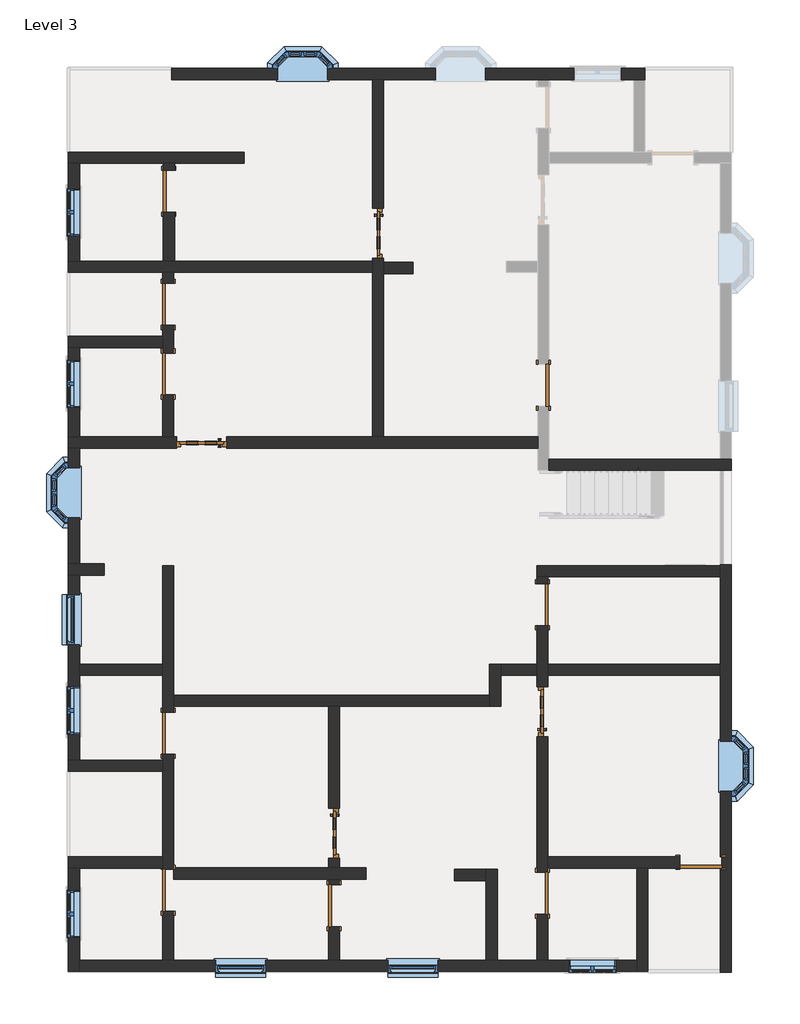
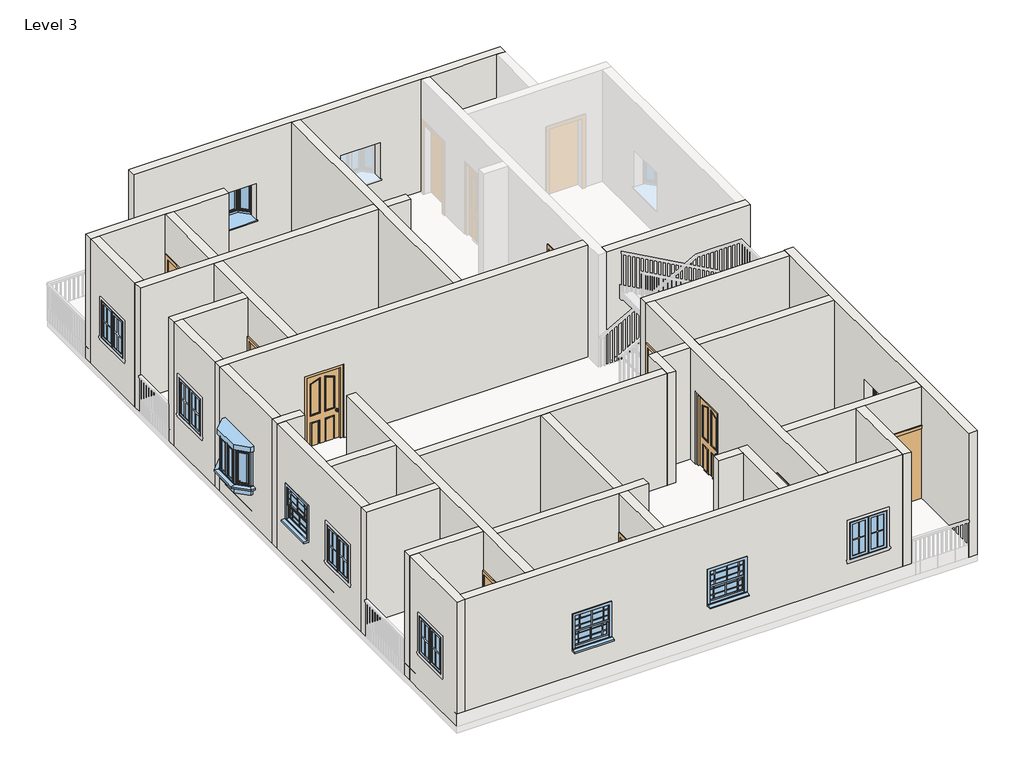
# One storey, part 1 of 4: 34 walls, 14 doors, 11 windows.
# Revit data of these elements (continued)
# Elements 15, 17, 18 (IfcWall, "Generic - 4.5\"") (continued)
#   Top Constraint = Level 4
#   Materials on its faces: "Default Wall", "Brick, Soldier Course"
# Elements 16, 20, 27, 31 (IfcWall, "Generic - 4.5\"")
#   Top Offset = 0' - 0"
#   Base Offset = 0' - 0"
#   wall height = 10' - 0"
#   Phase Created = New Construction
#   Base Constraint = Level 3
#   Top Constraint = Level 4
#   Materials on its faces: "Default Wall", "Parking Stripe"
# Elements 19, 21, 22, 30 (IfcWall, "Generic - 4.5\"")
#   Top Offset = 0' - 0"
#   Base Offset = 0' - 0"
#   wall height = 10' - 0"
#   Phase Created = New Construction
#   Base Constraint = Level 3
#   Top Constraint = Level 4
#   Materials on its faces: "Default Wall", "Earth"
# Element 23 (IfcWall, "Generic - 4.5\"")
#   Top Offset = 0' - 0"
#   Base Offset = 0' - 0"
#   wall height = 10' - 0"
#   Phase Created = New Construction
#   Base Constraint = Level 3
#   Top Constraint = Level 4
#   Materials on its faces: "Default Wall", "Door - Frame/Mullion"
# Elements 24, 25, 26, 29, 32, 33, 34, 35, 36, 37, 38, 39, 40 (IfcWall, "Generic - 4.5\"")
#   Top Offset = 0' - 0"
#   Base Offset = 0' - 0"
#   wall height = 10' - 0"
#   Phase Created = New Construction
#   Base Constraint = Level 3
#   Top Constraint = Level 4
#   Materials on its faces: "Default Wall"
# Element 28 (IfcWall, "Generic - 4.5\"")
#   Top Offset = 0' - 0"
#   Base Offset = 0' - 0"
#   wall height = 10' - 0"
#   Phase Created = New Construction
#   Base Constraint = Level 3
#   Top Constraint = Level 4
#   Materials on its faces: "Default Wall", "Parking Stripe", "Cherry"
# Elements 41, 46 (IfcWall, "Generic - 9\"")
#   Top Offset = 0' - 0"
#   Base Offset = 0' - 0"
#   wall height = 10' - 0"
#   Phase Created = New Construction
#   Base Constraint = Level 3
#   Top Constraint = Level 4
#   Materials on its faces: "Default Wall", "Parking Stripe", "Cherry"
# Element 42 (IfcWall, "Generic - 9\"")
#   Top Offset = 0' - 0"
#   Base Offset = 0' - 0"
#   wall height = 10' - 0"
#   Phase Created = New Construction
#   Base Constraint = Level 3
#   Top Constraint = Level 4
#   Materials on its faces: "Default Wall", "Door - Frame/Mullion", "Parking Stripe"
# Element 43 (IfcWall, "Generic - 9\"")
#   Top Offset = 0' - 0"
#   Base Offset = 0' - 0"
#   wall height = 10' - 0"
#   Phase Created = New Construction
#   Base Constraint = Level 3
#   Top Constraint = Level 4
#   Materials on its faces: "Default Wall", "Parking Stripe"
# Elements 44, 45, 48 (IfcWall, "Generic - 9\"")
#   Top Offset = 0' - 0"
#   Base Offset = 0' - 0"
#   wall height = 10' - 0"
#   Phase Created = New Construction
#   Base Constraint = Level 3
#   Top Constraint = Level 4
#   Materials on its faces: "Default Wall", "Earth"
# Element 47 (IfcWall, "Generic - 9\"")
#   Top Offset = 0' - 0"
#   Base Offset = 0' - 0"
#   wall height = 10' - 0"
#   Phase Created = New Construction
#   Base Constraint = Level 3
#   Top Constraint = Level 4
#   Materials on its faces: "Default Wall", "Cherry"
# Element 49 (IfcWindow, "910x910mm")
#   Mark = "31"
#   Phase Created = New Construction
#   Materials on its faces: "Window Frame", "Glass"
# Element 50 (IfcWindow, "910x910mm")
#   Mark = "34"
#   Phase Created = New Construction
#   Materials on its faces: "Window Frame", "Glass"
# Element 51 (IfcWindow, "910x910mm")
#   Mark = "35"
#   Phase Created = New Construction
#   Materials on its faces: "Window Frame", "Glass"
# Element 52 (IfcWindow, "Window-Casement-Double : 34\" x 36\"")
#   Mark = "40"
#   Window Inset = 0' - 0"
#   Interior Wall Closure = 0' - 2 1/4"
#   Frame Extension = 0' - 0 1/4"
#   Exterior Wall Closure = 0' - 1 1/4"
#   Interior Trim Visibility = yes
#   Exterior Trim Visibility = yes
#   Phase Created = New Construction
#   Materials on its faces: "Wood - Stained", "Glass", "Clad - White"
# Element 53 (IfcWindow, "Window-Casement-Double : 34\" x 36\"")
#   Mark = "41"
#   Window Inset = 0' - 0"
#   Interior Wall Closure = 0' - 2 1/4"
#   Frame Extension = 0' - 0 1/4"
#   Exterior Wall Closure = 0' - 1 1/4"
#   Interior Trim Visibility = yes
#   Exterior Trim Visibility = yes
#   Phase Created = New Construction
#   Materials on its faces: "Wood - Stained", "Glass", "Clad - White"
# Element 54 (IfcWindow, "Window-Casement-Double : 34\" x 36\"")
#   Mark = "43"
#   Window Inset = 0' - 0"
#   Interior Wall Closure = 0' - 2 1/4"
#   Frame Extension = 0' - 0 1/4"
#   Exterior Wall Closure = 0' - 1 1/4"
#   Interior Trim Visibility = yes
#   Exterior Trim Visibility = yes
#   Phase Created = New Construction
#   Materials on its faces: "Wood - Stained", "Glass", "Clad - White"
# Element 55 (IfcWindow, "Window-Casement-Double : 34\" x 36\"")
#   Mark = "44"
#   Window Inset = 0' - 0"
#   Interior Wall Closure = 0' - 2 1/4"
#   Frame Extension = 0' - 0 1/4"
#   Exterior Wall Closure = 0' - 1 1/4"
#   Interior Trim Visibility = yes
#   Exterior Trim Visibility = yes
#   Phase Created = New Construction
#   Materials on its faces: "Wood - Stained", "Glass", "Clad - White"
# Element 56 (IfcWindow, "Window-Casement-Double : 34\" x 36\"")
#   Mark = "45"
#   Window Inset = 0' - 0"
#   Interior Wall Closure = 0' - 2 1/4"
#   Frame Extension = 0' - 0 1/4"
#   Exterior Wall Closure = 0' - 1 1/4"
#   Interior Trim Visibility = yes
#   Exterior Trim Visibility = yes
#   Phase Created = New Construction
#   Materials on its faces: "Wood - Stained", "Glass", "Clad - White"
# Element 57 (IfcWindow, "Windows_Sash_w-Bars_1 : 910x910mm")
#   Mark = "36"
#   Phase Created = New Construction
#   Materials on its faces: "Window Frame", "Glass"
# Element 58 (IfcWindow, "Windows_Sash_w-Bars_1 : 910x910mm")
#   Mark = "37"
#   Phase Created = New Construction
#   Materials on its faces: "Window Frame", "Glass"
# Element 59 (IfcWindow, "Windows_Sash_w-Bars_1 : 910x910mm")
#   Mark = "38"
#   Phase Created = New Construction
#   Materials on its faces: "Window Frame", "Glass"
# Materials
#   "Door - Glazing": colour RGB 0 0 255, transparency 0.75
#   "Door - Panel": class "Wood", colour RGB 210 159 95, transparency 0, Cost = 0
#   "Door - Frame/Mullion": class "Wood", colour RGB 212 179 113, transparency 0
#   "Door - Handle": colour RGB 247 247 247, transparency 0
#   "Door - Frame": colour RGB 118 70 51, transparency 0, Cost = 0
#   "Window Frame": colour RGB 249 249 249, transparency 0
#   "Glass": class "Glass", colour RGB 0 128 192, transparency 0.75, Description = "Soda Lime Glass", Cost = 0
#   "Wood - Stained": class "Wood", colour RGB 224 178 126, transparency 0, Cost = 0
#   "Clad - White": class "Wood", colour RGB 242 242 238, transparency 0, Cost = 0
#   "Default Wall": colour RGB 128 128 128, transparency 0, Cost = 0
#   "Brick, Soldier Course": class "Masonry", colour RGB 170 98 104, transparency 0, Description = "Common brick soldier coursed", Cost = 0
#   "Parking Stripe": class "Paint", colour RGB 250 250 91, transparency 0, Cost = 0
#   "Earth": class "Generic", colour RGB 97 75 62, transparency 0, Description = "Soil", Cost = 0
#   "Cherry": class "Wood", colour RGB 226 177 128, transparency 0, Description = "Prunus Serotina", Cost = 0
